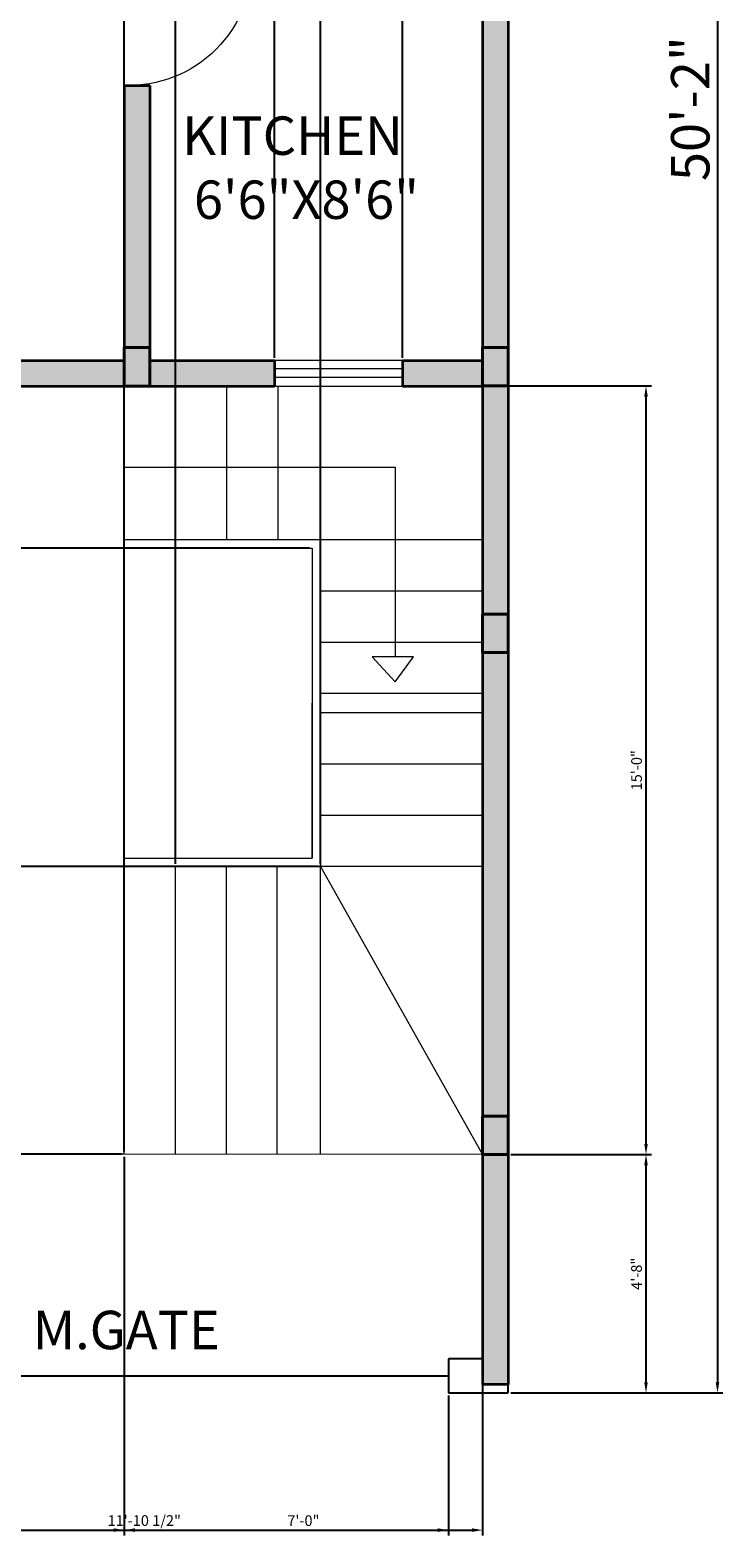
# Model space of a CAD drawing. Units: inches. Extents: x 5276 to 5736, y 3292 to 3966.
# Tile 2 of 3: x 5574 to 5736, y 3292 to 3646. Entities that reach past the tile are written whole.
import ezdxf

# ---------------------------------------------------------------- set-up
doc = ezdxf.new("R2010")
doc.units = ezdxf.units.IN
for name, color, linetype, lineweight in [('A-ANNO-DIMS', 2, 'Continuous', 18), ('A-ANNO-TEXT', 7, 'Continuous', 18), ('A-AREA-IDEN', 7, 'Continuous', 18), ('A-COLS', 7, 'Continuous', 40), ('A-DOOR', 3, 'Continuous', 18), ('A-FLOR-STRS', 9, 'Continuous', 18), ('A-GLAZ', 4, 'Continuous', 18), ('A-ROOF', 9, 'Continuous', 18), ('A-SITE-GATE', 7, 'Continuous', 25), ('A-WALL', 7, 'Continuous', 35)]:
    doc.layers.add(name, color=color, linetype=linetype, lineweight=lineweight)
doc.layers.add('A-COLS-PATT', color=244, linetype='Continuous', lineweight=13, true_color=0x991b1e)
doc.layers.add('A-WALL-PATT', color=141, linetype='Continuous', lineweight=13, true_color=0xadddf7)
doc.styles.get("Standard").update_dxf_attribs({"font": 'arial.ttf'})
doc.dimstyles.new('ISO-25', dxfattribs={"dimtxt": 2.5, "dimasz": 2.5, "dimexe": 1.25, "dimexo": 0.625, "dimtad": 1, "dimlunit": 3, "dimtxsty": 'Standard', "dimcen": 2.5, "dimadec": 0, "dimazin": 0, "dimtfac": 1, "dimtmove": 0, "dimatfit": 3, "dimfxl": 1, "dimarcsym": 0})

# ---------------------------------------------------------------- blocks, each defined once
blk = doc.blocks.new('*D17')
at = {"layer": 'A-ANNO-DIMS', "color": 0, "lineweight": -2, "transparency": 16777216}
for p, q in [((5686.75, 3928.25), (5736.45, 3928.25)), ((5735.2, 3925.75), (5735.2, 3328.75)), ((5686.75, 3326.25), (5736.45, 3326.25))]:
    blk.add_line(p, q, dxfattribs=at)
at = {"layer": 'A-ANNO-DIMS', "color": 0, "transparency": 16777216}
for points in [[(5734.78, 3925.75), (5735.62, 3925.75), (5735.2, 3928.25)], [(5734.78, 3328.75), (5735.62, 3328.75), (5735.2, 3326.25)]]:
    blk.add_solid(points, dxfattribs=at)
at = {"layer": 'Defpoints', "color": 0, "transparency": 16777216}
for p in [(5686.13, 3928.25), (5686.13, 3326.25), (5735.2, 3326.25)]:
    blk.add_point(p, dxfattribs=at)
at = {"layer": 'A-ANNO-DIMS', "color": 0, "transparency": 16777216, "insert": (5729.98, 3627.25), "char_height": 9, "attachment_point": 5, "rotation": 90}
blk.add_mtext('50\'-2"', dxfattribs=at)
blk = doc.blocks.new('PIER-6X9')
for p, q in [((0, 9), (6, 9)), ((0, 0), (0, 9)), ((6, 9), (6, 0)), ((6, 0), (0, 0))]:
    blk.add_line(p, q)
blk = doc.blocks.new('DOOR-SWING-30')
for p, q in [((0, 30), (-2, 30)), ((-2, 30), (-2, 0)), ((0, 0), (0, 30)), ((-2, 0), (0, 0))]:
    blk.add_line(p, q)
blk.add_arc((-1, 1), 29.02, 88.0251, 181.9749)
blk = doc.blocks.new('*D32')
at = {"layer": 'A-ANNO-DIMS', "color": 0, "lineweight": -2, "transparency": 16777216}
for p, q in [((5529.5, 3325.62), (5529.5, 3292.85)), ((5672.13, 3325.62), (5672.13, 3292.85)), ((5532, 3294.1), (5669.63, 3294.1))]:
    blk.add_line(p, q, dxfattribs=at)
at = {"layer": 'A-ANNO-DIMS', "color": 0, "transparency": 16777216}
for points in [[(5532, 3294.52), (5532, 3293.68), (5529.5, 3294.1)], [(5669.63, 3294.52), (5669.63, 3293.68), (5672.13, 3294.1)]]:
    blk.add_solid(points, dxfattribs=at)
at = {"layer": 'Defpoints', "color": 0, "transparency": 16777216}
for p in [(5529.5, 3326.25), (5672.13, 3326.25), (5672.13, 3294.1)]:
    blk.add_point(p, dxfattribs=at)
at = {"layer": 'A-ANNO-DIMS', "color": 0, "transparency": 16777216, "insert": (5600.82, 3296.02), "char_height": 2.5, "attachment_point": 5}
blk.add_mtext('11\'-10 1/2"', dxfattribs=at)
blk = doc.blocks.new('*D34')
at = {"layer": 'A-ANNO-DIMS', "color": 0, "lineweight": -2, "transparency": 16777216}
for p, q in [((5686.77, 3382.13), (5719.69, 3382.13)), ((5718.44, 3328.75), (5718.44, 3379.63)), ((5686.75, 3326.25), (5719.69, 3326.25))]:
    blk.add_line(p, q, dxfattribs=at)
at = {"layer": 'A-ANNO-DIMS', "color": 0, "transparency": 16777216}
for points in [[(5718.02, 3379.63), (5718.86, 3379.63), (5718.44, 3382.13)], [(5718.02, 3328.75), (5718.86, 3328.75), (5718.44, 3326.25)]]:
    blk.add_solid(points, dxfattribs=at)
at = {"layer": 'Defpoints', "color": 0, "transparency": 16777216}
for p in [(5686.14, 3382.13), (5718.44, 3382.13), (5686.13, 3326.25)]:
    blk.add_point(p, dxfattribs=at)
at = {"layer": 'A-ANNO-DIMS', "color": 0, "transparency": 16777216, "insert": (5716.54, 3354.19), "char_height": 2.5, "attachment_point": 5, "rotation": 90}
blk.add_mtext('4\'-8"', dxfattribs=at)
blk = doc.blocks.new('*D35')
at = {"layer": 'A-ANNO-DIMS', "color": 0, "lineweight": -2, "transparency": 16777216}
for p, q in [((5680.75, 3562.25), (5719.69, 3562.25)), ((5718.44, 3384.63), (5718.44, 3559.75)), ((5686.77, 3382.13), (5719.69, 3382.13))]:
    blk.add_line(p, q, dxfattribs=at)
at = {"layer": 'A-ANNO-DIMS', "color": 0, "transparency": 16777216}
for points in [[(5718.02, 3559.75), (5718.86, 3559.75), (5718.44, 3562.25)], [(5718.02, 3384.63), (5718.86, 3384.63), (5718.44, 3382.13)]]:
    blk.add_solid(points, dxfattribs=at)
at = {"layer": 'Defpoints', "color": 0, "transparency": 16777216}
for p in [(5680.13, 3562.25), (5718.44, 3562.25), (5686.14, 3382.13)]:
    blk.add_point(p, dxfattribs=at)
at = {"layer": 'A-ANNO-DIMS', "color": 0, "transparency": 16777216, "insert": (5716.54, 3472.19), "char_height": 2.5, "attachment_point": 5, "rotation": 90}
blk.add_mtext('15\'-0"', dxfattribs=at)
blk = doc.blocks.new('*D41')
at = {"layer": 'A-ANNO-DIMS', "color": 0, "lineweight": -2, "transparency": 16777216}
for p, q in [((5476.13, 3382.87), (5476.13, 3961.65)), ((5596.12, 3382.87), (5596.12, 3961.65)), ((5478.63, 3960.4), (5593.62, 3960.4))]:
    blk.add_line(p, q, dxfattribs=at)
at = {"layer": 'A-ANNO-DIMS', "color": 0, "transparency": 16777216}
for points in [[(5478.63, 3960.82), (5478.63, 3959.98), (5476.13, 3960.4)], [(5593.62, 3960.82), (5593.62, 3959.98), (5596.12, 3960.4)]]:
    blk.add_solid(points, dxfattribs=at)
at = {"layer": 'Defpoints', "color": 0, "transparency": 16777216}
for p in [(5596.12, 3960.4), (5476.13, 3382.25), (5596.12, 3382.25)]:
    blk.add_point(p, dxfattribs=at)
at = {"layer": 'A-ANNO-DIMS', "color": 0, "transparency": 16777216, "insert": (5536.12, 3962.3), "char_height": 2.5, "attachment_point": 5}
blk.add_mtext('10\'-0"', dxfattribs=at)
blk = doc.blocks.new('*D42')
at = {"layer": 'A-ANNO-DIMS', "color": 0, "lineweight": -2, "transparency": 16777216}
for p, q in [((5539.19, 3381.62), (5539.19, 3292.85)), ((5596.12, 3381.62), (5596.12, 3292.85)), ((5541.69, 3294.1), (5593.62, 3294.1))]:
    blk.add_line(p, q, dxfattribs=at)
at = {"layer": 'A-ANNO-DIMS', "color": 0, "transparency": 16777216}
for points in [[(5541.69, 3294.52), (5541.69, 3293.68), (5539.19, 3294.1)], [(5593.62, 3294.52), (5593.62, 3293.68), (5596.12, 3294.1)]]:
    blk.add_solid(points, dxfattribs=at)
at = {"layer": 'Defpoints', "color": 0, "transparency": 16777216}
for p in [(5539.19, 3382.25), (5596.12, 3382.25), (5596.12, 3294.1)]:
    blk.add_point(p, dxfattribs=at)
at = {"layer": 'A-ANNO-DIMS', "color": 0, "transparency": 16777216, "insert": (5567.65, 3296), "char_height": 2.5, "attachment_point": 5}
blk.add_mtext('4\'-9"', dxfattribs=at)
blk = doc.blocks.new('*D43')
at = {"layer": 'A-ANNO-DIMS', "color": 0, "lineweight": -2, "transparency": 16777216}
for p, q in [((5596.12, 3381.62), (5596.12, 3292.85)), ((5680.13, 3381.51), (5680.13, 3292.85)), ((5598.62, 3294.1), (5677.63, 3294.1))]:
    blk.add_line(p, q, dxfattribs=at)
at = {"layer": 'A-ANNO-DIMS', "color": 0, "transparency": 16777216}
for points in [[(5598.62, 3294.52), (5598.62, 3293.68), (5596.12, 3294.1)], [(5677.63, 3294.52), (5677.63, 3293.68), (5680.13, 3294.1)]]:
    blk.add_solid(points, dxfattribs=at)
at = {"layer": 'Defpoints', "color": 0, "transparency": 16777216}
for p in [(5596.12, 3382.25), (5680.13, 3382.13), (5680.13, 3294.1)]:
    blk.add_point(p, dxfattribs=at)
at = {"layer": 'A-ANNO-DIMS', "color": 0, "transparency": 16777216, "insert": (5638.12, 3296), "char_height": 2.5, "attachment_point": 5}
blk.add_mtext('7\'-0"', dxfattribs=at)
blk = doc.blocks.new('*D44')
at = {"layer": 'A-ANNO-DIMS', "color": 0, "lineweight": -2, "transparency": 16777216}
for p, q in [((5642.17, 3450.24), (5642.17, 3961.65)), ((5680.13, 3450.24), (5680.13, 3961.65)), ((5644.67, 3960.4), (5677.63, 3960.4))]:
    blk.add_line(p, q, dxfattribs=at)
at = {"layer": 'A-ANNO-DIMS', "color": 0, "transparency": 16777216}
for points in [[(5644.67, 3960.82), (5644.67, 3959.98), (5642.17, 3960.4)], [(5677.63, 3960.82), (5677.63, 3959.98), (5680.13, 3960.4)]]:
    blk.add_solid(points, dxfattribs=at)
at = {"layer": 'Defpoints', "color": 0, "transparency": 16777216}
for p in [(5680.13, 3960.4), (5642.17, 3449.62), (5680.13, 3449.62)]:
    blk.add_point(p, dxfattribs=at)
at = {"layer": 'A-ANNO-DIMS', "color": 0, "transparency": 16777216, "insert": (5661.15, 3962.3), "char_height": 2.5, "attachment_point": 5}
blk.add_mtext('3\'-2"', dxfattribs=at)
blk = doc.blocks.new('*D45')
at = {"layer": 'A-ANNO-DIMS', "color": 0, "lineweight": -2, "transparency": 16777216}
for p, q in [((5639.55, 3524.24), (5280.73, 3524.24)), ((5281.98, 3521.74), (5281.98, 3452.12)), ((5641.55, 3449.62), (5280.73, 3449.62))]:
    blk.add_line(p, q, dxfattribs=at)
at = {"layer": 'A-ANNO-DIMS', "color": 0, "transparency": 16777216}
for points in [[(5281.56, 3521.74), (5282.39, 3521.74), (5281.98, 3524.24)], [(5281.56, 3452.12), (5282.39, 3452.12), (5281.98, 3449.62)]]:
    blk.add_solid(points, dxfattribs=at)
at = {"layer": 'Defpoints', "color": 0, "transparency": 16777216}
for p in [(5640.17, 3524.24), (5281.98, 3449.62), (5642.17, 3449.62)]:
    blk.add_point(p, dxfattribs=at)
at = {"layer": 'A-ANNO-DIMS', "color": 0, "transparency": 16777216, "insert": (5280.06, 3486.93), "char_height": 2.5, "attachment_point": 5, "rotation": 90}
blk.add_mtext('6\'-2 1/2"', dxfattribs=at)
blk = doc.blocks.new('*D46')
at = {"layer": 'A-ANNO-DIMS', "color": 0, "lineweight": -2, "transparency": 16777216}
for p, q in [((5595.49, 3449.62), (5280.73, 3449.62)), ((5281.98, 3384.75), (5281.98, 3447.12)), ((5595.49, 3382.25), (5280.73, 3382.25))]:
    blk.add_line(p, q, dxfattribs=at)
at = {"layer": 'A-ANNO-DIMS', "color": 0, "transparency": 16777216}
for points in [[(5281.56, 3447.12), (5282.39, 3447.12), (5281.98, 3449.62)], [(5281.56, 3384.75), (5282.39, 3384.75), (5281.98, 3382.25)]]:
    blk.add_solid(points, dxfattribs=at)
at = {"layer": 'Defpoints', "color": 0, "transparency": 16777216}
for p in [(5281.98, 3449.62), (5596.12, 3449.62), (5596.12, 3382.25)]:
    blk.add_point(p, dxfattribs=at)
at = {"layer": 'A-ANNO-DIMS', "color": 0, "transparency": 16777216, "insert": (5280.06, 3415.93), "char_height": 2.5, "attachment_point": 5, "rotation": 90}
blk.add_mtext('5\'-7 1/2"', dxfattribs=at)
blk = doc.blocks.new('*D47')
at = {"layer": 'A-ANNO-DIMS', "color": 0, "lineweight": -2, "transparency": 16777216}
for p, q in [((5596.12, 3450.24), (5596.12, 3961.65)), ((5608.12, 3450.24), (5608.12, 3961.65)), ((5598.62, 3960.4), (5605.62, 3960.4))]:
    blk.add_line(p, q, dxfattribs=at)
at = {"layer": 'A-ANNO-DIMS', "color": 0, "transparency": 16777216}
for points in [[(5598.62, 3960.82), (5598.62, 3959.98), (5596.12, 3960.4)], [(5605.62, 3960.82), (5605.62, 3959.98), (5608.12, 3960.4)]]:
    blk.add_solid(points, dxfattribs=at)
at = {"layer": 'Defpoints', "color": 0, "transparency": 16777216}
for p in [(5608.12, 3960.4), (5596.12, 3449.62), (5608.12, 3449.62)]:
    blk.add_point(p, dxfattribs=at)
at = {"layer": 'A-ANNO-DIMS', "color": 0, "transparency": 16777216, "insert": (5602.12, 3962.3), "char_height": 2.5, "attachment_point": 5}
blk.add_mtext('1\'-0"', dxfattribs=at)
blk = doc.blocks.new('*D52')
at = {"layer": 'A-ANNO-DIMS', "color": 0, "lineweight": -2, "transparency": 16777216}
for p, q in [((5631.38, 3568.87), (5631.38, 3961.65)), ((5661.38, 3568.87), (5661.38, 3961.65)), ((5633.88, 3960.4), (5658.88, 3960.4))]:
    blk.add_line(p, q, dxfattribs=at)
at = {"layer": 'A-ANNO-DIMS', "color": 0, "transparency": 16777216}
for points in [[(5633.88, 3960.82), (5633.88, 3959.98), (5631.38, 3960.4)], [(5658.88, 3960.82), (5658.88, 3959.98), (5661.38, 3960.4)]]:
    blk.add_solid(points, dxfattribs=at)
at = {"layer": 'Defpoints', "color": 0, "transparency": 16777216}
for p in [(5661.38, 3960.4), (5631.38, 3568.25), (5661.38, 3568.25)]:
    blk.add_point(p, dxfattribs=at)
at = {"layer": 'A-ANNO-DIMS', "color": 0, "transparency": 16777216, "insert": (5646.38, 3962.3), "char_height": 2.5, "attachment_point": 5}
blk.add_mtext('2\'-6"', dxfattribs=at)

msp = doc.modelspace()

# ---------------------------------------------------------------- hatches: boundary and pattern name
at = {"layer": 'A-COLS-PATT'}
h = msp.add_hatch(color=256, dxfattribs=at)
h.dxf.hatch_style = 1
h.paths.add_polyline_path([(5320.127, 3874.381), (5314.129, 3874.381), (5314.129, 3865.381), (5320.127, 3865.381)])
h.paths.add_polyline_path([(5500.127, 3874.249), (5494.136, 3874.249), (5494.136, 3865.268), (5500.127, 3865.268)])
h.paths.add_polyline_path([(5500.127, 3733.242), (5494.138, 3733.242), (5494.138, 3724.249), (5500.127, 3724.249)])
h.paths.add_polyline_path([(5569.096, 3928.221), (5560.096, 3928.221), (5560.096, 3922.249), (5560.127, 3922.249), (5566.127, 3922.23), (5566.127, 3922.249), (5569.096, 3922.249)])
h.paths.add_polyline_path([(5686.127, 3747.872), (5680.127, 3747.872), (5680.127, 3731.687), (5686.127, 3731.687)])
h.paths.add_polyline_path([(5503.112, 3676.236), (5494.127, 3676.236), (5494.127, 3670.249), (5503.112, 3670.249)])
h.paths.add_polyline_path([(5320.127, 3514.161), (5314.167, 3514.161), (5314.167, 3505.161), (5320.127, 3505.161)])
h.paths.add_polyline_path([(5320.127, 3391.305), (5314.138, 3391.305), (5314.138, 3382.305), (5320.127, 3382.305)])
h.paths.add_polyline_path([(5476.116, 3391.239), (5470.127, 3391.239), (5470.127, 3382.249), (5476.116, 3382.249)])
h.paths.add_polyline_path([(5476.1, 3508.238), (5470.127, 3508.238), (5470.127, 3499.238), (5476.1, 3499.238)])
h.paths.add_polyline_path([(5359.148, 3568.249), (5350.148, 3568.249), (5350.148, 3562.297), (5359.148, 3562.297)])
h.paths.add_polyline_path([(5476.127, 3568.222), (5467.137, 3568.222), (5467.137, 3562.249), (5476.127, 3562.249)])
h.paths.add_polyline_path([(5602.119, 3571.238), (5596.127, 3571.238), (5596.127, 3562.249), (5602.119, 3562.249)])
h.paths.add_polyline_path([(5686.112, 3571.26), (5680.127, 3571.26), (5680.127, 3568.249), (5680.112, 3562.26), (5686.112, 3562.26)])
h.paths.add_polyline_path([(5686.094, 3508.787), (5680.127, 3508.787), (5680.127, 3499.787), (5686.094, 3499.787)])
h = msp.add_hatch(color=256, dxfattribs=at)
h.dxf.hatch_style = 1
h.paths.add_polyline_path([(5686.127, 3391.131), (5680.144, 3391.131), (5680.144, 3382.131), (5686.127, 3382.131)])
at = {"layer": 'A-WALL-PATT'}
h = msp.add_hatch(color=256, dxfattribs=at)
h.dxf.hatch_style = 1
h.paths.add_polyline_path([(5560.096, 3928.249), (5314.127, 3928.249), (5314.127, 3874.381), (5320.127, 3874.381), (5320.127, 3922.249), (5560.096, 3922.249)])
h.paths.add_polyline_path([(5500.127, 3865.268), (5494.127, 3865.268), (5494.127, 3733.242), (5500.127, 3733.242)])
h.paths.add_polyline_path([(5644.696, 3874.249), (5566.127, 3874.249), (5566.127, 3891.071), (5560.127, 3891.071), (5560.127, 3868.249), (5644.696, 3868.249)])
h.paths.add_polyline_path([(5686.127, 3928.249), (5569.096, 3928.249), (5569.096, 3922.249), (5680.127, 3922.249), (5680.127, 3874.262), (5686.127, 3874.262)])
h.paths.add_polyline_path([(5686.127, 3865.262), (5680.127, 3865.262), (5680.127, 3756.872), (5686.127, 3756.872)])
h.paths.add_polyline_path([(5393.929, 3874.249), (5320.129, 3874.249), (5320.129, 3868.249), (5393.929, 3868.249)])
h.paths.add_polyline_path([(5459.929, 3874.249), (5441.929, 3874.249), (5441.929, 3868.249), (5459.929, 3868.249)])
h.paths.add_polyline_path([(5447.929, 3730.249), (5338.127, 3730.249), (5338.127, 3724.249), (5356.127, 3724.249), (5356.127, 3628.249), (5344.74, 3628.249), (5344.74, 3622.249), (5356.127, 3622.249), (5356.127, 3598.249), (5362.127, 3598.249), (5362.127, 3724.249), (5447.929, 3724.249)])
h.paths.add_polyline_path([(5320.127, 3865.381), (5314.127, 3865.381), (5314.127, 3514.249), (5320.127, 3514.249), (5320.127, 3568.249)])
h.paths.add_polyline_path([(5686.127, 3722.687), (5680.127, 3722.687), (5680.127, 3676.249), (5503.112, 3676.249), (5503.112, 3670.249), (5596.127, 3670.249), (5596.127, 3662.687), (5602.127, 3662.687), (5602.127, 3670.249), (5680.127, 3670.249), (5680.127, 3571.26), (5686.127, 3571.26)])
h.paths.add_polyline_path([(5596.119, 3568.249), (5536.127, 3568.249), (5536.127, 3562.249), (5543.142, 3562.249), (5596.119, 3562.249)])
h.paths.add_polyline_path([(5602.127, 3632.687), (5596.127, 3632.687), (5596.127, 3571.238), (5602.127, 3571.238)])
h.paths.add_polyline_path([(5631.383, 3568.249), (5602.127, 3568.249), (5602.127, 3562.249), (5631.383, 3562.249)])
h.paths.add_polyline_path([(5680.112, 3568.249), (5661.383, 3568.249), (5661.383, 3562.249), (5680.112, 3562.249)])
h.paths.add_polyline_path([(5686.127, 3562.26), (5680.127, 3562.26), (5680.127, 3508.787), (5686.127, 3508.787)])
h.paths.add_polyline_path([(5686.127, 3499.787), (5680.127, 3499.787), (5680.127, 3391.131), (5686.127, 3391.131)])
h.paths.add_polyline_path([(5686.127, 3382.131), (5680.127, 3382.131), (5680.127, 3328.249), (5686.127, 3328.249)])
h.paths.add_polyline_path([(5320.127, 3505.161), (5314.127, 3505.161), (5314.127, 3391.305), (5320.127, 3391.305)])
h.paths.add_polyline_path([(5344.127, 3388.249), (5320.138, 3388.249), (5320.138, 3382.249), (5344.127, 3382.249)])
h.paths.add_polyline_path([(5428.127, 3388.249), (5392.127, 3388.249), (5392.127, 3382.249), (5428.127, 3382.249)])
h.paths.add_polyline_path([(5476.127, 3499.238), (5470.127, 3499.238), (5470.127, 3397.332), (5470.127, 3391.239), (5476.127, 3391.239), (5476.127, 3397.332)])
h.paths.add_polyline_path([(5446.127, 3517.875), (5440.127, 3517.875), (5440.127, 3514.249), (5356.127, 3514.249), (5356.127, 3528.065), (5350.127, 3528.065), (5350.127, 3508.249), (5446.127, 3508.249)])
h.paths.add_polyline_path([(5356.127, 3562.249), (5350.127, 3562.249), (5350.127, 3552.065), (5356.127, 3552.065)])
h.paths.add_polyline_path([(5467.137, 3568.249), (5359.148, 3568.249), (5359.148, 3562.249), (5440.127, 3562.249), (5440.127, 3547.875), (5446.127, 3547.875), (5446.127, 3562.249), (5467.137, 3562.249)])

# ---------------------------------------------------------------- linework, layer by layer
at = {"layer": 'A-FLOR-STRS'}
for p, q in [((5596.119, 3562.238), (5596.119, 3524.238)), ((5608.119, 3562.238), (5608.119, 3526.238)), ((5620.119, 3562.238), (5620.119, 3526.238)), ((5632.119, 3562.238), (5632.119, 3526.238)), ((5596.119, 3543.238), (5659.627, 3543.238)), ((5659.627, 3543.238), (5659.627, 3498.787)), ((5596.119, 3526.238), (5680.127, 3526.238)), ((5596.119, 3524.238), (5640.172, 3524.238)), ((5640.172, 3524.238), (5640.172, 3451.615)), ((5642.172, 3526.238), (5642.172, 3449.615)), ((5642.172, 3514.238), (5680.127, 3514.238)), ((5642.172, 3502.238), (5680.127, 3502.238)), ((5659.627, 3498.787), (5654.274, 3498.787)), ((5654.274, 3498.787), (5659.627, 3492.902)), ((5659.627, 3492.902), (5663.941, 3498.787)), ((5663.941, 3498.787), (5659.627, 3498.787)), ((5640.172, 3451.615), (5640.172, 3487.927)), ((5642.172, 3490.238), (5680.127, 3490.238)), ((5642.172, 3449.615), (5642.172, 3487.927)), ((5680.127, 3485.615), (5642.172, 3485.615)), ((5680.127, 3473.615), (5642.172, 3473.615)), ((5680.127, 3461.615), (5642.172, 3461.615)), ((5596.119, 3382.249), (5596.119, 3451.615)), ((5596.119, 3451.615), (5640.172, 3451.615)), ((5642.172, 3449.615), (5596.119, 3449.615)), ((5596.119, 3449.615), (5642.172, 3449.615)), ((5608.119, 3382.249), (5608.119, 3449.615)), ((5608.119, 3382.249), (5608.119, 3449.615)), ((5620.119, 3382.249), (5620.119, 3449.615)), ((5631.952, 3382.199), (5631.952, 3449.615)), ((5642.172, 3449.615), (5642.172, 3449.615)), ((5680.127, 3449.615), (5642.172, 3449.615)), ((5642.172, 3382.184), (5642.172, 3449.615)), ((5642.172, 3449.615), (5680.127, 3382.131)), ((5680.144, 3382.131), (5596.119, 3382.249))]:
    msp.add_line(p, q, dxfattribs=at)
at = {"layer": 'A-GLAZ'}
for p, q in [((5661.383, 3568.249), (5631.383, 3568.249)), ((5631.383, 3568.249), (5631.383, 3562.249)), ((5661.383, 3566.249), (5631.383, 3566.249)), ((5661.383, 3562.249), (5661.383, 3568.249)), ((5661.383, 3564.249), (5631.383, 3564.249)), ((5631.383, 3562.249), (5661.383, 3562.249))]:
    msp.add_line(p, q, dxfattribs=at)
at = {"layer": 'A-ROOF'}
msp.add_line((5596.119, 3382.249), (5539.189, 3382.249), dxfattribs=at)
at = {"layer": 'A-SITE-GATE'}
for p, q in [((5680.127, 3334.249), (5672.127, 3334.249)), ((5680.127, 3334.249), (5672.127, 3334.249)), ((5672.127, 3334.249), (5672.127, 3326.249)), ((5529.504, 3330.249), (5672.127, 3330.249)), ((5672.127, 3326.249), (5686.127, 3326.249)), ((5686.127, 3326.249), (5686.127, 3328.249))]:
    msp.add_line(p, q, dxfattribs=at)
at = {"layer": 'A-WALL'}
for p, q in [((5686.127, 3928.249), (5686.127, 3328.249)), ((5680.127, 3670.249), (5680.127, 3568.249)), ((5596.127, 3632.687), (5602.127, 3632.687)), ((5596.127, 3632.687), (5596.127, 3562.249)), ((5602.127, 3632.687), (5602.127, 3562.249)), ((5536.127, 3568.249), (5596.127, 3568.249)), ((5602.127, 3568.249), (5631.383, 3568.249)), ((5602.127, 3568.249), (5631.383, 3568.249)), ((5631.383, 3568.249), (5631.383, 3562.249)), ((5661.383, 3568.249), (5661.383, 3562.249)), ((5661.383, 3568.249), (5680.127, 3568.249)), ((5661.383, 3568.249), (5662.127, 3568.249)), ((5543.142, 3562.249), (5631.383, 3562.249)), ((5661.383, 3562.249), (5680.127, 3562.249)), ((5680.127, 3562.249), (5680.127, 3328.249)), ((5686.127, 3328.249), (5680.127, 3328.249))]:
    msp.add_line(p, q, dxfattribs=at)

# ---------------------------------------------------------------- block references
at = {"layer": 'A-COLS', "rotation": 180}
for p in [(5602.119, 3571.238), (5686.112, 3571.26), (5686.094, 3508.787), (5686.144, 3391.131)]:
    msp.add_blockref('PIER-6X9', p, dxfattribs=at)
at = {"layer": 'A-DOOR', "extrusion": (0, 0, -1), "zscale": -1, "rotation": 89.99999999999642}
msp.add_blockref('DOOR-SWING-30', (-5596.127, 3662.687), dxfattribs=at)

# ---------------------------------------------------------------- texts
at = {"layer": 'A-ANNO-TEXT', "insert": (5571.902, 3345.503), "char_height": 9, "attachment_point": 1}
msp.add_mtext_dynamic_manual_height_columns(' M.GATE', width=110.27411, gutter_width=12.5, heights=[0], dxfattribs=at)
at = {"layer": 'A-AREA-IDEN', "insert": (5606.965, 3625.419), "char_height": 9, "attachment_point": 1}
msp.add_mtext_dynamic_manual_height_columns(' KITCHEN\\P  6\'6"X8\'6"', width=110.27411, gutter_width=12.5, heights=[0], dxfattribs=at)

# ---------------------------------------------------------------- dimensions: what is measured, and where the dimension line sits
at = {"layer": 'A-ANNO-DIMS'}
for base, p1, p2, picture, middle in [((5596.119, 3960.399), (5476.127, 3382.249), (5596.119, 3382.249), '*D41', (5536.123, 3962.301)), ((5608.119, 3960.399), (5596.119, 3449.615), (5608.119, 3449.615), '*D47', (5602.119, 3962.301)), ((5661.383, 3960.399), (5631.383, 3568.249), (5661.383, 3568.249), '*D52', (5646.383, 3962.301)), ((5680.127, 3960.399), (5642.172, 3449.615), (5680.127, 3449.615), '*D44', (5661.149, 3962.301)), ((5596.119, 3294.099), (5539.189, 3382.249), (5596.119, 3382.249), '*D42', (5567.654, 3296.001)), ((5680.127, 3294.099), (5596.119, 3382.249), (5680.127, 3382.131), '*D43', (5638.123, 3296.001)), ((5672.127, 3294.099), (5529.504, 3326.249), (5672.127, 3326.249), '*D32', (5600.816, 3296.017))]:
    dim = msp.add_linear_dim(base=base, p1=p1, p2=p2, dimstyle='ISO-25', override={"dimdec": 1, "dimlfac": 1, "dimrnd": 0, "dimzin": 1, "dimdsep": 46, "dimlunit": 4, "dimfrac": 2}, dxfattribs=at)
    dim.commit()
    dim.dimension.update_dxf_attribs({"geometry": picture, "text_midpoint": middle})
for base, p1, p2, override, picture, middle in [((5735.2, 3326.249), (5686.127, 3928.249), (5686.127, 3326.249), {"dimtxt": 9, "dimclrd": 0, "dimclre": 0, "dimclrt": 0}, '*D17', (5729.98, 3627.249)), ((5718.44, 3562.249), (5686.144, 3382.131), (5680.127, 3562.249), {"dimdec": 1, "dimlfac": 1, "dimrnd": 0, "dimzin": 1, "dimdsep": 46, "dimlunit": 4, "dimfrac": 2}, '*D35', (5716.539, 3472.19)), ((5281.977, 3449.615), (5640.172, 3524.238), (5642.172, 3449.615), {"dimdec": 1, "dimlfac": 1, "dimrnd": 0, "dimzin": 1, "dimdsep": 46, "dimlunit": 4, "dimfrac": 2}, '*D45', (5280.059, 3486.927)), ((5281.977, 3449.615), (5596.119, 3382.249), (5596.119, 3449.615), {"dimdec": 1, "dimlfac": 1, "dimrnd": 0, "dimzin": 1, "dimdsep": 46, "dimlunit": 4, "dimfrac": 2}, '*D46', (5280.059, 3415.932)), ((5718.44, 3382.131), (5686.127, 3326.249), (5686.144, 3382.131), {"dimdec": 1, "dimlfac": 1, "dimrnd": 0, "dimzin": 1, "dimdsep": 46, "dimlunit": 4, "dimfrac": 2}, '*D34', (5716.539, 3354.19))]:
    dim = msp.add_linear_dim(base=base, p1=p1, p2=p2, angle=90, dimstyle='ISO-25', override=override, dxfattribs=at)
    dim.commit()
    dim.dimension.update_dxf_attribs({"geometry": picture, "text_midpoint": middle})

doc.saveas('drawing.dxf')
